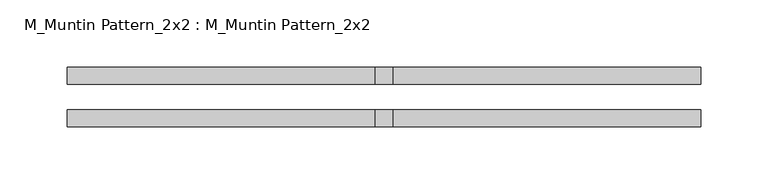
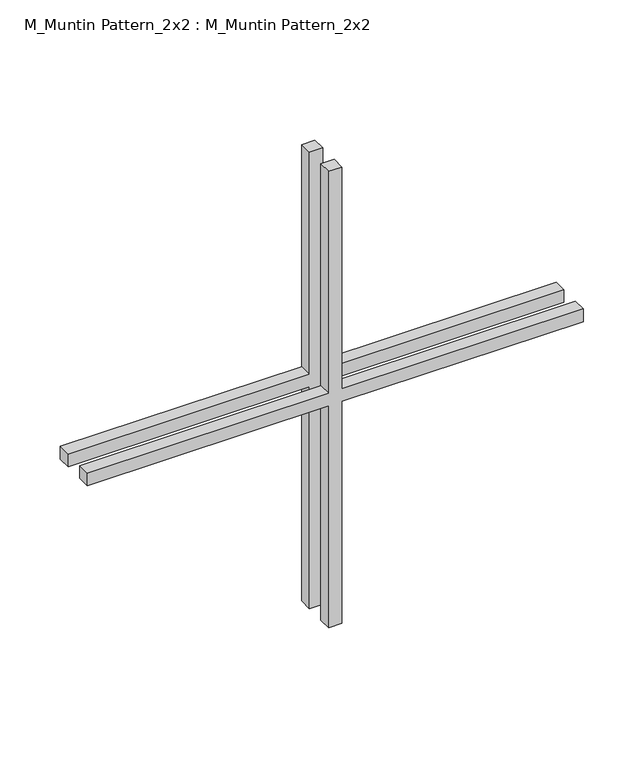
"""IFC4 building model written with IfcOpenShell, lengths in millimetres: proxy geometry, M_Muntin Pattern_2x2 : M_Muntin Pattern_2x2."""

from ifc_helpers import new_model, si_unit, frame, origin, place, context, project, spatial, polyline, outline, extrude, source, transform, mapped, element, save


def m_muntin_pattern_2x2_m_muntin_pattern_2x2_6a19bea2(model_context):
    return source(origin(), model_context, "Body", "SweptSolid", [
        extrude(outline(polyline([(236.5, -6.35), (236.5, -236.5375), (223.8, -236.5375), (223.8, -6.35), (0.0, -6.35), (0.0, 6.35), (223.8, 6.35), (223.8, 236.5375), (236.5, 236.5375), (236.5, 6.35), (460.3, 6.35), (460.3, -6.35), (236.5, -6.35)])), frame((0.0, -22.225, 0.0), z_axis=(0.0, 1.0, 0.0), x_axis=(0.0, 0.0, 1.0)), (0.0, 0.0, 1.0), 12.7),
        extrude(outline(polyline([(236.5, -6.35), (236.5, -236.5375), (223.8, -236.5375), (223.8, -6.35), (0.0, -6.35), (0.0, 6.35), (223.8, 6.35), (223.8, 236.5375), (236.5, 236.5375), (236.5, 6.35), (460.3, 6.35), (460.3, -6.35), (236.5, -6.35)])), frame((0.0, 9.525, 0.0), z_axis=(0.0, 1.0, 0.0), x_axis=(0.0, 0.0, 1.0)), (0.0, 0.0, 1.0), 12.7),
    ])


if __name__ == "__main__":
    model = new_model("IFC4")
    model_context = context("Model", 3, world=origin())
    ifc_project = project(units=[si_unit("LENGTHUNIT", "METRE", prefix="MILLI")], contexts=[model_context])
    site = spatial("IfcSite", under=ifc_project)
    building = spatial("IfcBuilding", under=site)
    placement = place(None, origin())
    m_muntin_pattern_2x2_m_muntin_pattern_2x2_shape = m_muntin_pattern_2x2_m_muntin_pattern_2x2_6a19bea2(model_context)
    element("IfcBuildingElementProxy", 1, Name="M_Muntin Pattern_2x2 : M_Muntin Pattern_2x2", ObjectType="M_Muntin Pattern_2x2 : M_Muntin Pattern_2x2", at=placement, inside=building, context=model_context, shape_type="MappedRepresentation", body=[
        mapped(m_muntin_pattern_2x2_m_muntin_pattern_2x2_shape, transform((0.0, 0.0, 0.0), x_axis=(1.0, 0.0, 0.0), y_axis=(0.0, 1.0, 0.0), z_axis=(0.0, 0.0, 1.0))),
    ])
    save(model, "model.ifc")

# Revit data of these elements
# Type "M_Muntin Pattern_2x2 : M_Muntin Pattern_2x2"
#   Width [instance default] = 3' - 11.24409"
#   Thickness = 0' - 0 1/2"
#   Height [instance default] = 3' - 11.24409"
#   Distance = 0' - 0 3/4"
#   Interior Material [instance default] = none
#   Exterior Material [instance default] = none
#   Default Elevation = 0
# Element 1 (IfcBuildingElementProxy, "M_Muntin Pattern_2x2 : M_Muntin Pattern_2x2")
#   Width = 1' - 6 5/8"
#   Height = 1' - 6.12205"
#   Interior Material = Wood - Stained
#   Exterior Material = Clad - White
#   Materials on its faces: "Clad - White", "Wood - Stained"
# Materials
#   "Clad - White": class "Wood", colour RGB 242 242 238, transparency 0, Cost = 0
#   "Wood - Stained": class "Wood", colour RGB 227 170 128, transparency 0, Cost = 0
